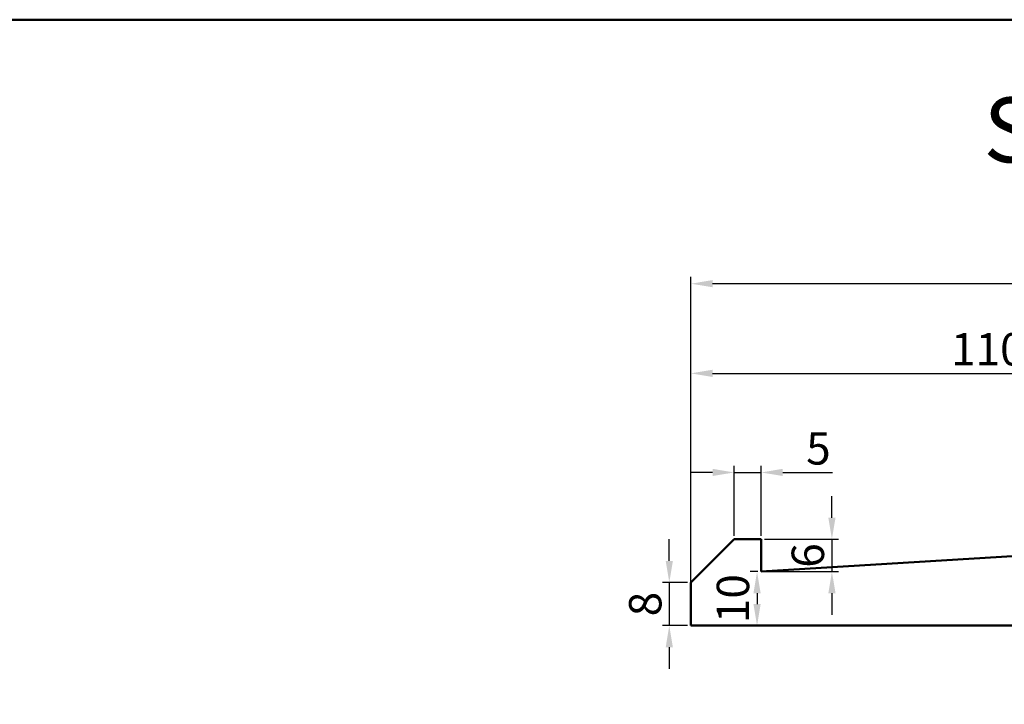
# Model space of a CAD drawing. Units: millimetres. Extents: x -25 to 763, y -62 to 306.
# Tile 4 of 7: x 258 to 440, y 179 to 306. Entities that reach past the tile are written whole.
import ezdxf

# ---------------------------------------------------------------- set-up
doc = ezdxf.new("R2010")
doc.units = ezdxf.units.MM
doc.header["$LTSCALE"] = 0.5
for name, color, linetype, lineweight in [('M-DIMS', 2, 'Continuous', 25), ('M-OUTL', 7, 'Continuous', 50), ('M-TTLB', 7, 'Continuous', 50)]:
    doc.layers.add(name, color=color, linetype=linetype, lineweight=lineweight)
doc.styles.get("Standard").update_dxf_attribs({"font": 'arial.ttf'})
doc.dimstyles.new('ISO-25', dxfattribs={"dimtxt": 6, "dimasz": 4, "dimexe": 1.25, "dimexo": 0.625, "dimtad": 1, "dimtoh": 1, "dimdec": 1, "dimtxsty": 'Standard', "dimcen": 2.5, "dimadec": 0, "dimazin": 0, "dimtfac": 1, "dimtdec": 1, "dimtmove": 0, "dimatfit": 3, "dimfxl": 1, "dimarcsym": 0})

# ---------------------------------------------------------------- blocks, each defined once
blk = doc.blocks.new('*D62')
at = {"layer": 'Defpoints', "color": 0, "ltscale": 0.5, "transparency": 16777216}
for p in [(492.09, 240.22), (382.09, 194.54), (492.09, 194.54)]:
    blk.add_point(p, dxfattribs=at)
at = {"layer": 'M-DIMS', "color": 0, "lineweight": -2, "ltscale": 0.5, "transparency": 16777216}
for p, q in [((382.09, 195.17), (382.09, 241.47)), ((492.09, 195.17), (492.09, 241.47)), ((386.09, 240.22), (488.09, 240.22))]:
    blk.add_line(p, q, dxfattribs=at)
at = {"layer": 'M-DIMS', "color": 0, "ltscale": 0.5, "transparency": 16777216}
for points in [[(386.09, 240.89), (386.09, 239.55), (382.09, 240.22)], [(488.09, 240.89), (488.09, 239.55), (492.09, 240.22)]]:
    blk.add_solid(points, dxfattribs=at)
at = {"layer": 'M-DIMS', "color": 0, "ltscale": 0.5, "transparency": 16777216, "insert": (437.09, 243.91), "char_height": 6, "attachment_point": 5}
blk.add_mtext('110', dxfattribs=at)
blk = doc.blocks.new('*D63')
at = {"layer": 'Defpoints', "color": 0, "ltscale": 0.5, "transparency": 16777216}
for p in [(395.09, 221.86), (390.09, 209.48), (395.09, 209.48)]:
    blk.add_point(p, dxfattribs=at)
at = {"layer": 'M-DIMS', "color": 0, "lineweight": -2, "ltscale": 0.5, "transparency": 16777216}
for p, q in [((390.09, 210.1), (390.09, 223.11)), ((395.09, 210.1), (395.09, 223.11)), ((386.09, 221.86), (382.09, 221.86)), ((390.09, 221.86), (395.09, 221.86)), ((399.09, 221.86), (408.32, 221.86))]:
    blk.add_line(p, q, dxfattribs=at)
at = {"layer": 'M-DIMS', "color": 0, "ltscale": 0.5, "transparency": 16777216}
for points in [[(386.09, 222.53), (386.09, 221.2), (390.09, 221.86)], [(399.09, 222.53), (399.09, 221.2), (395.09, 221.86)]]:
    blk.add_solid(points, dxfattribs=at)
at = {"layer": 'M-DIMS', "color": 0, "ltscale": 0.5, "transparency": 16777216, "insert": (405.7, 225.54), "char_height": 6, "attachment_point": 5}
blk.add_mtext('5', dxfattribs=at)
blk = doc.blocks.new('*D64')
at = {"layer": 'Defpoints', "color": 0, "ltscale": 0.5, "transparency": 16777216}
for p in [(395.09, 209.48), (395.09, 203.48), (408.2, 203.48)]:
    blk.add_point(p, dxfattribs=at)
at = {"layer": 'M-DIMS', "color": 0, "lineweight": -2, "ltscale": 0.5, "transparency": 16777216}
for p, q in [((408.2, 213.48), (408.2, 217.48)), ((395.72, 209.48), (409.45, 209.48)), ((408.2, 209.48), (408.2, 203.48)), ((395.72, 203.48), (409.45, 203.48)), ((408.2, 199.48), (408.2, 195.48))]:
    blk.add_line(p, q, dxfattribs=at)
at = {"layer": 'M-DIMS', "color": 0, "ltscale": 0.5, "transparency": 16777216}
for points in [[(407.54, 213.48), (408.87, 213.48), (408.2, 209.48)], [(407.54, 199.48), (408.87, 199.48), (408.2, 203.48)]]:
    blk.add_solid(points, dxfattribs=at)
at = {"layer": 'M-DIMS', "color": 0, "ltscale": 0.5, "transparency": 16777216, "insert": (404.52, 206.48), "char_height": 6, "attachment_point": 5, "rotation": 90}
blk.add_mtext('6', dxfattribs=at)
blk = doc.blocks.new('*D65')
at = {"layer": 'Defpoints', "color": 0, "ltscale": 0.5, "transparency": 16777216}
for p in [(395.09, 203.48), (394.33, 193.48), (395.71, 193.48)]:
    blk.add_point(p, dxfattribs=at)
at = {"layer": 'M-DIMS', "color": 0, "lineweight": -2, "ltscale": 0.5, "transparency": 16777216}
for p, q in [((394.47, 203.48), (393.08, 203.48)), ((394.33, 199.48), (394.33, 197.48)), ((395.08, 193.48), (393.08, 193.48))]:
    blk.add_line(p, q, dxfattribs=at)
at = {"layer": 'M-DIMS', "color": 0, "ltscale": 0.5, "transparency": 16777216}
for points in [[(393.66, 199.48), (395, 199.48), (394.33, 203.48)], [(393.66, 197.48), (395, 197.48), (394.33, 193.48)]]:
    blk.add_solid(points, dxfattribs=at)
at = {"layer": 'M-DIMS', "color": 0, "ltscale": 0.5, "transparency": 16777216, "insert": (390.64, 198.48), "char_height": 6, "attachment_point": 5, "rotation": 90}
blk.add_mtext('10', dxfattribs=at)
blk = doc.blocks.new('*D66')
at = {"layer": 'Defpoints', "color": 0, "ltscale": 0.5, "transparency": 16777216}
for p in [(382.09, 201.48), (378.07, 193.48), (382.09, 193.48)]:
    blk.add_point(p, dxfattribs=at)
at = {"layer": 'M-DIMS', "color": 0, "lineweight": -2, "ltscale": 0.5, "transparency": 16777216}
for p, q in [((378.07, 205.48), (378.07, 209.48)), ((381.47, 201.48), (376.82, 201.48)), ((378.07, 201.48), (378.07, 193.48)), ((381.47, 193.48), (376.82, 193.48)), ((378.07, 189.48), (378.07, 185.48))]:
    blk.add_line(p, q, dxfattribs=at)
at = {"layer": 'M-DIMS', "color": 0, "ltscale": 0.5, "transparency": 16777216}
for points in [[(377.41, 205.48), (378.74, 205.48), (378.07, 201.48)], [(377.41, 189.48), (378.74, 189.48), (378.07, 193.48)]]:
    blk.add_solid(points, dxfattribs=at)
at = {"layer": 'M-DIMS', "color": 0, "ltscale": 0.5, "transparency": 16777216, "insert": (374.39, 197.48), "char_height": 6, "attachment_point": 5, "rotation": 90}
blk.add_mtext('8', dxfattribs=at)
blk = doc.blocks.new('*D67')
at = {"layer": 'Defpoints', "color": 0, "ltscale": 0.5, "transparency": 16777216}
for p in [(382.09, 256.83), (674.09, 201.48), (382.09, 197.48)]:
    blk.add_point(p, dxfattribs=at)
at = {"layer": 'M-DIMS', "color": 0, "lineweight": -2, "ltscale": 0.5, "transparency": 16777216}
for p, q in [((382.09, 198.1), (382.09, 258.08)), ((674.09, 202.1), (674.09, 258.08)), ((670.09, 256.83), (386.09, 256.83))]:
    blk.add_line(p, q, dxfattribs=at)
at = {"layer": 'M-DIMS', "color": 0, "ltscale": 0.5, "transparency": 16777216}
for points in [[(386.09, 257.5), (386.09, 256.17), (382.09, 256.83)], [(670.09, 257.5), (670.09, 256.17), (674.09, 256.83)]]:
    blk.add_solid(points, dxfattribs=at)
at = {"layer": 'M-DIMS', "color": 0, "ltscale": 0.5, "transparency": 16777216, "insert": (528.09, 260.52), "char_height": 6, "attachment_point": 5}
blk.add_mtext('292', dxfattribs=at)

msp = doc.modelspace()

# ---------------------------------------------------------------- linework, layer by layer
at = {"layer": 'M-OUTL', "ltscale": 0.5}
for p, q in [((382.09, 201.48), (390.09, 209.48)), ((390.09, 209.48), (395.09, 209.48)), ((395.09, 209.48), (395.09, 203.48)), ((395.09, 203.48), (492.09, 209.48)), ((382.09, 193.48), (382.09, 201.48)), ((626.59, 193.48), (382.09, 193.48))]:
    msp.add_line(p, q, dxfattribs=at)
at = {"layer": 'M-TTLB', "ltscale": 0.5}
msp.add_lwpolyline([(229.22, 305.74), (763.29, 305.74), (763.29, -62.45), (229.22, -62.45)], close=True, dxfattribs=at)

# ---------------------------------------------------------------- texts
at = {"layer": 'M-TTLB', "ltscale": 0.5, "insert": (403.69, 291.33), "char_height": 12, "attachment_point": 1}
msp.add_mtext_dynamic_manual_height_columns('\\pxqc;SAFETY VALVE ASSEMBLY', width=257.4414, gutter_width=12.5, heights=[0], dxfattribs=at)

# ---------------------------------------------------------------- dimensions: what is measured, and where the dimension line sits
at = {"layer": 'M-DIMS', "ltscale": 0.5}
for base, p1, p2, picture, middle in [((382.09, 256.83), (674.09, 201.48), (382.09, 197.48), '*D67', (528.09, 260.52)), ((492.09, 240.22), (382.09, 194.54), (492.09, 194.54), '*D62', (437.09, 243.91)), ((395.09, 221.86), (390.09, 209.48), (395.09, 209.48), '*D63', (405.7, 225.54))]:
    dim = msp.add_linear_dim(base=base, p1=p1, p2=p2, dimstyle='ISO-25', override={"dimclrd": 0, "dimclre": 0, "dimclrt": 0}, dxfattribs=at)
    dim.commit()
    dim.dimension.update_dxf_attribs({"geometry": picture, "text_midpoint": middle})
for base, p1, p2, picture, middle in [((408.2, 203.48), (395.09, 209.48), (395.09, 203.48), '*D64', (404.52, 206.48)), ((378.07, 193.48), (382.09, 201.48), (382.09, 193.48), '*D66', (374.39, 197.48)), ((394.33, 193.48), (395.09, 203.48), (395.71, 193.48), '*D65', (390.64, 198.48))]:
    dim = msp.add_linear_dim(base=base, p1=p1, p2=p2, angle=90, dimstyle='ISO-25', override={"dimclrd": 0, "dimclre": 0, "dimclrt": 0}, dxfattribs=at)
    dim.commit()
    dim.dimension.update_dxf_attribs({"geometry": picture, "text_midpoint": middle})

doc.saveas('drawing.dxf')
